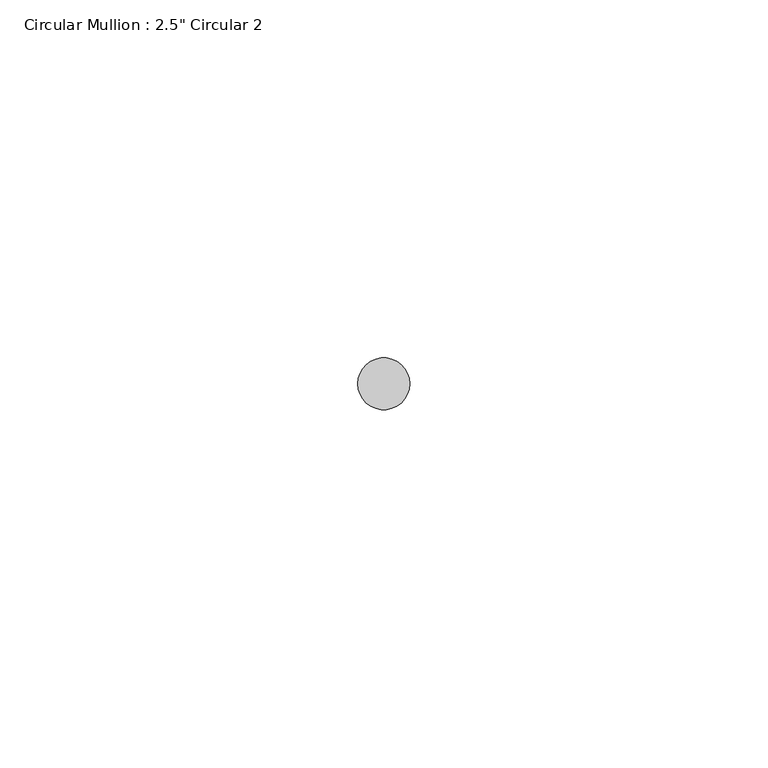
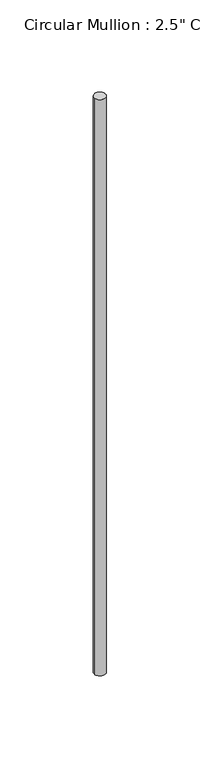
"""IFC4 building model written with IfcOpenShell, lengths in millimetres: member geometry."""

from ifc_helpers import new_model, si_unit, point, frame, origin, origin_2d, place, context, project, spatial, circle_curve, trimmed, segment, composite_curve, outline, extrude, source, transform, mapped, element, save


def member_b3cb6624(model_context):
    return source(origin(), model_context, "Body", "SweptSolid", [
        extrude(outline(composite_curve([segment(trimmed(circle_curve(origin_2d(), 3.6195), [point((3.6195, 0.0))], [point((-3.6195, 0.0))], False, "CARTESIAN"), True, "CONTINUOUS"), segment(trimmed(circle_curve(origin_2d(), 3.6195), [point((-3.6195, 0.0))], [point((3.6195, 0.0))], False, "CARTESIAN"), True, "CONTINUOUS")], self_intersect=False)), frame((0.0, 0.0, -387.35), z_axis=(0.0, 0.0, 1.0), x_axis=(1.0, 0.0, 0.0)), (0.0, 0.0, 1.0), 387.35),
    ])


if __name__ == "__main__":
    model = new_model("IFC4")
    model_context = context("Model", 3, world=origin())
    ifc_project = project(units=[si_unit("LENGTHUNIT", "METRE", prefix="MILLI")], contexts=[model_context])
    site = spatial("IfcSite", under=ifc_project)
    building = spatial("IfcBuilding", under=site)
    placement = place(None, origin())
    member_shape = member_b3cb6624(model_context)
    element("IfcMember", 1, ObjectType="Circular Mullion : 2.5\" Circular 2", at=placement, inside=building, context=model_context, shape_type="MappedRepresentation", body=[
        mapped(member_shape, transform((0.0, 0.0, 0.0), x_axis=(1.0, 0.0, 0.0), y_axis=(0.0, 1.0, 0.0), z_axis=(0.0, 0.0, 1.0))),
    ])
    save(model, "model.ifc")

# Revit data of these elements
# Type "Circular Mullion : 2.5\" Circular 2"
#   built-in parameter 1007350 = 0.011875 (stored number, unit not read)
# Element 1 (IfcMember, "Circular Mullion : 2.5\" Circular 2")
#   Materials on its faces: "Aluminum"
# Materials
#   "Aluminum": class "Metal", colour RGB 247 247 247, transparency 0, Description = "Aluminum 6061", Cost = 0
